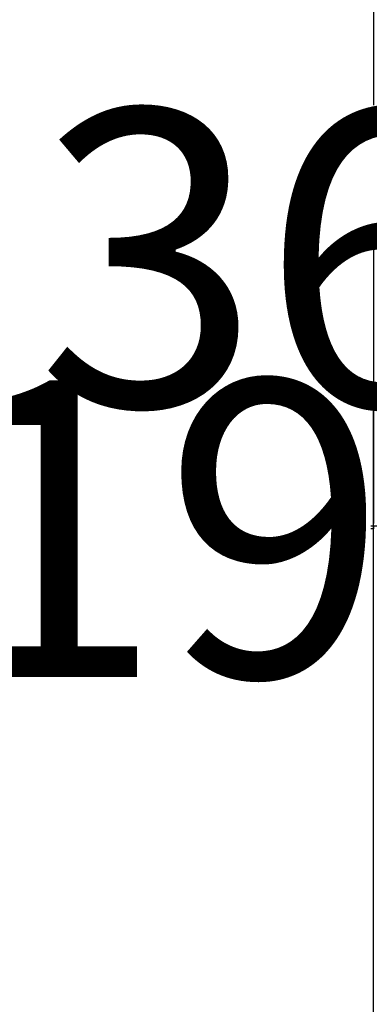
# Model space of a CAD drawing. Units: inches. Extents: x 305 to 776, y 38 to 479.
# Tile 3 of 14: x 349 to 372, y 199 to 265. Entities that reach past the tile are written whole.
import ezdxf

# ---------------------------------------------------------------- set-up
doc = ezdxf.new("R2010")
doc.units = ezdxf.units.IN
doc.header["$MEASUREMENT"] = 0
doc.layers.add('A-ANNO-DIMS', color=2, linetype='Continuous', lineweight=18)
doc.styles.get("Standard").update_dxf_attribs({"font": 'arial.ttf'})
doc.dimstyles.get("Standard").update_dxf_attribs({"dimtxt": 20, "dimasz": 0.18, "dimexe": 0.18, "dimexo": 0.0625, "dimgap": 0.09, "dimtad": 0, "dimtih": 1, "dimtoh": 1, "dimdec": 4, "dimzin": 0, "dimdsep": 46, "dimtxsty": 'Standard', "dimcen": 0.09, "dimadec": 0, "dimazin": 0, "dimtfac": 1, "dimtdec": 4, "dimtofl": 0, "dimtmove": 0, "dimatfit": 3, "dimfxl": 1, "dimtolj": 1, "dimtzin": 0, "dimarcsym": 0})

# ---------------------------------------------------------------- blocks, each defined once
blk = doc.blocks.new('*D33')
at = {"layer": 'A-ANNO-DIMS', "color": 0, "lineweight": -2, "transparency": 16777216}
for p, q in [((440.927, 307.949), (449.29, 307.949)), ((449.11, 307.769), (449.11, 290.896)), ((449.11, 253.161), (449.11, 270.034)), ((440.927, 252.981), (449.29, 252.981))]:
    blk.add_line(p, q, dxfattribs=at)
at = {"layer": 'A-ANNO-DIMS', "color": 0, "transparency": 16777216}
for points in [[(449.08, 307.769), (449.14, 307.769), (449.11, 307.949)], [(449.08, 253.161), (449.14, 253.161), (449.11, 252.981)]]:
    blk.add_solid(points, dxfattribs=at)
at = {"layer": 'Defpoints', "color": 0, "transparency": 16777216}
for p in [(440.864, 307.949), (449.11, 307.949), (440.864, 252.981)]:
    blk.add_point(p, dxfattribs=at)
at = {"layer": 'A-ANNO-DIMS', "color": 0, "transparency": 16777216, "insert": (449.11, 280.465), "char_height": 20, "attachment_point": 5}
blk.add_mtext('\\A1;DINING SET 55', dxfattribs=at)
blk = doc.blocks.new('*D46')
at = {"layer": 'A-ANNO-DIMS', "color": 0, "lineweight": -2, "transparency": 16777216}
for p, q in [((390.57, 429.382), (372.451, 429.382)), ((372.631, 429.202), (372.631, 259.69)), ((372.631, 69.562), (372.631, 239.074)), ((390.57, 69.382), (372.451, 69.382))]:
    blk.add_line(p, q, dxfattribs=at)
at = {"layer": 'A-ANNO-DIMS', "color": 0, "transparency": 16777216}
for points in [[(372.601, 429.202), (372.661, 429.202), (372.631, 429.382)], [(372.601, 69.562), (372.661, 69.562), (372.631, 69.382)]]:
    blk.add_solid(points, dxfattribs=at)
at = {"layer": 'Defpoints', "color": 0, "transparency": 16777216}
for p in [(372.631, 429.382), (390.633, 429.382), (390.633, 69.382)]:
    blk.add_point(p, dxfattribs=at)
at = {"layer": 'A-ANNO-DIMS', "color": 0, "transparency": 16777216, "insert": (372.631, 249.382), "char_height": 20, "attachment_point": 5}
blk.add_mtext('\\A1;360', dxfattribs=at)
blk = doc.blocks.new('*D74')
at = {"layer": 'A-ANNO-DIMS', "color": 0, "lineweight": -2, "transparency": 16777216}
for p, q in [((399.57, 250.482), (372.451, 250.482)), ((372.631, 250.302), (372.631, 231.472)), ((404.07, 231.292), (372.451, 231.292)), ((372.631, 231.292), (372.631, 231.112)), ((372.631, 231.112), (372.451, 231.112))]:
    blk.add_line(p, q, dxfattribs=at)
at = {"layer": 'A-ANNO-DIMS', "color": 0, "transparency": 16777216}
for points in [[(372.601, 250.302), (372.661, 250.302), (372.631, 250.482)], [(372.601, 231.472), (372.661, 231.472), (372.631, 231.292)]]:
    blk.add_solid(points, dxfattribs=at)
at = {"layer": 'Defpoints', "color": 0, "transparency": 16777216}
for p in [(399.633, 250.482), (372.631, 231.292), (404.133, 231.292)]:
    blk.add_point(p, dxfattribs=at)
at = {"layer": 'A-ANNO-DIMS', "color": 0, "transparency": 16777216, "insert": (339.537, 231.112), "char_height": 20, "attachment_point": 5}
blk.add_mtext('\\A1;19.19', dxfattribs=at)

msp = doc.modelspace()

# ---------------------------------------------------------------- dimensions: what is measured, and where the dimension line sits
at = {"layer": 'A-ANNO-DIMS'}
for base, p1, p2, override, picture, middle in [((372.6314, 429.382), (390.6329, 69.382), (390.6329, 429.382), {"dimdec": 0, "dimlfac": 1, "dimrnd": 0, "dimzin": 0, "dimdsep": 46, "dimlunit": 2}, '*D46', (372.6314, 249.382)), ((372.6314, 231.2915), (399.6329, 250.4819), (404.1329, 231.2915), {"dimdec": 2, "dimlfac": 1, "dimrnd": 0, "dimzin": 0, "dimdsep": 46, "dimlunit": 2}, '*D74', (339.5374, 231.1115))]:
    dim = msp.add_linear_dim(base=base, p1=p1, p2=p2, angle=90, dimstyle='Standard', override=override, dxfattribs=at)
    dim.commit()
    dim.dimension.update_dxf_attribs({"geometry": picture, "text_midpoint": middle})
dim = msp.add_linear_dim(base=(449.1096, 307.9493), p1=(440.8644, 252.9815), p2=(440.8644, 307.9493), angle=90, text='DINING SET <>', dimstyle='Standard', override={"dimdec": 0, "dimlfac": 1, "dimrnd": 0, "dimzin": 0, "dimdsep": 46, "dimlunit": 2}, dxfattribs=at)
dim.commit()
dim.dimension.update_dxf_attribs({"geometry": '*D33', "text_midpoint": (449.1096, 280.4654)})

doc.saveas('drawing.dxf')
